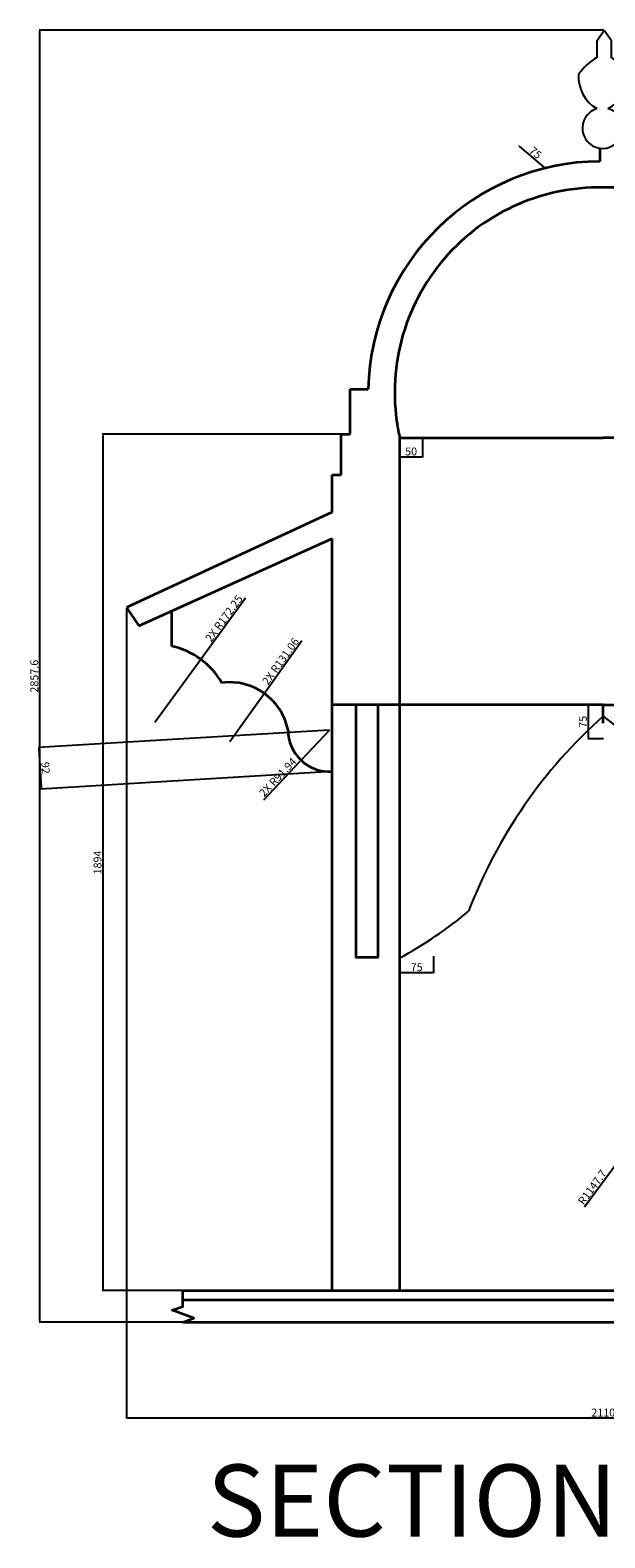
# Model space of a CAD drawing. Units: millimetres. Extents: x 498 to 8860, y -426 to 8717.
# Tile 5 of 9: x 527 to 1798, y 3606 to 6941. Entities that reach past the tile are written whole.
import ezdxf

# ---------------------------------------------------------------- set-up
doc = ezdxf.new("R2010")
doc.units = ezdxf.units.MM
for name, color, linetype, lineweight in [('A-ANNO-DIMS', 2, 'Continuous', 18), ('A-ANNO-TEXT', 3, 'Continuous', 18), ('A-DETL', 7, 'Continuous', 25), ('A-SECT', 7, 'Continuous', 35)]:
    doc.layers.add(name, color=color, linetype=linetype, lineweight=lineweight)
doc.styles.get("Standard").update_dxf_attribs({"font": 'arial.ttf'})
doc.dimstyles.new('ISO-25', dxfattribs={"dimtxt": 17.5, "dimasz": 2.5, "dimexe": 1.25, "dimexo": 0.625, "dimtad": 1, "dimdec": 0, "dimtxsty": 'Standard', "dimcen": 2.5, "dimadec": 0, "dimazin": 0, "dimtfac": 1, "dimtdec": 0, "dimtmove": 0, "dimatfit": 3, "dimfxl": 1, "dimarcsym": 0})

# ---------------------------------------------------------------- blocks, each defined once
blk = doc.blocks.new('*D29')
at = {"layer": 'A-ANNO-DIMS', "color": 0, "lineweight": -2, "transparency": 16777216}
for p, q in [((1344.7, 6038.9), (1344.7, 5996.1)), ((1394.8, 6038.9), (1394.8, 5996.1)), ((1347.2, 5997.3), (1392.3, 5997.3))]:
    blk.add_line(p, q, dxfattribs=at)
at = {"layer": 'A-ANNO-DIMS', "color": 0, "transparency": 16777216}
for points in [[(1347.2, 5997.8), (1347.2, 5996.9), (1344.7, 5997.3)], [(1392.3, 5997.8), (1392.3, 5996.9), (1394.8, 5997.3)]]:
    blk.add_solid(points, dxfattribs=at)
at = {"layer": 'Defpoints', "color": 0, "transparency": 16777216}
for p in [(1344.7, 6039.5), (1394.8, 6039.5), (1394.8, 5997.3)]:
    blk.add_point(p, dxfattribs=at)
at = {"layer": 'A-ANNO-DIMS', "color": 0, "transparency": 16777216, "insert": (1369.7, 6006.9), "char_height": 17.5, "attachment_point": 5}
blk.add_mtext('50', dxfattribs=at)
blk = doc.blocks.new('*D31')
at = {"layer": 'A-ANNO-DIMS', "color": 0, "lineweight": -2, "transparency": 16777216}
for p, q in [((1214.1, 6047.2), (686.4, 6047.2)), ((687.6, 6044.7), (687.6, 4155.7)), ((1194.1, 4153.2), (686.4, 4153.2))]:
    blk.add_line(p, q, dxfattribs=at)
at = {"layer": 'A-ANNO-DIMS', "color": 0, "transparency": 16777216}
for points in [[(687.2, 6044.7), (688, 6044.7), (687.6, 6047.2)], [(687.2, 4155.7), (688, 4155.7), (687.6, 4153.2)]]:
    blk.add_solid(points, dxfattribs=at)
at = {"layer": 'Defpoints', "color": 0, "transparency": 16777216}
for p in [(1214.7, 6047.2), (687.6, 4153.2), (1194.7, 4153.2)]:
    blk.add_point(p, dxfattribs=at)
at = {"layer": 'A-ANNO-DIMS', "color": 0, "transparency": 16777216, "insert": (678.1, 5100.2), "char_height": 17.5, "attachment_point": 5, "rotation": 90}
blk.add_mtext('1894', dxfattribs=at)
blk = doc.blocks.new('*D32')
at = {"layer": 'A-ANNO-DIMS', "color": 0, "lineweight": -2, "transparency": 16777216}
for p, q in [((1344.7, 4888.3), (1344.7, 4855.6)), ((1419.2, 4893), (1419.2, 4855.6)), ((1347.2, 4856.8), (1416.7, 4856.8))]:
    blk.add_line(p, q, dxfattribs=at)
at = {"layer": 'A-ANNO-DIMS', "color": 0, "transparency": 16777216}
for points in [[(1347.2, 4857.3), (1347.2, 4856.4), (1344.7, 4856.8)], [(1416.7, 4857.3), (1416.7, 4856.4), (1419.2, 4856.8)]]:
    blk.add_solid(points, dxfattribs=at)
at = {"layer": 'Defpoints', "color": 0, "transparency": 16777216}
for p in [(1344.7, 4889), (1419.2, 4893.6), (1419.2, 4856.8)]:
    blk.add_point(p, dxfattribs=at)
at = {"layer": 'A-ANNO-DIMS', "color": 0, "transparency": 16777216, "insert": (1382, 4866.4), "char_height": 17.5, "attachment_point": 5}
blk.add_mtext('75', dxfattribs=at)
blk = doc.blocks.new('*D34')
at = {"layer": 'A-ANNO-DIMS', "color": 0, "lineweight": -2, "transparency": 16777216}
for p, q in [((1794.1, 5448.8), (1760.3, 5448.8)), ((1761.6, 5446.3), (1761.6, 5376.5)), ((1795.1, 5374), (1760.3, 5374))]:
    blk.add_line(p, q, dxfattribs=at)
at = {"layer": 'A-ANNO-DIMS', "color": 0, "transparency": 16777216}
for points in [[(1761.2, 5446.3), (1762, 5446.3), (1761.6, 5448.8)], [(1761.2, 5376.5), (1762, 5376.5), (1761.6, 5374)]]:
    blk.add_solid(points, dxfattribs=at)
at = {"layer": 'Defpoints', "color": 0, "transparency": 16777216}
for p in [(1794.7, 5448.8), (1761.6, 5374), (1795.7, 5374)]:
    blk.add_point(p, dxfattribs=at)
at = {"layer": 'A-ANNO-DIMS', "color": 0, "transparency": 16777216, "insert": (1752, 5411.4), "char_height": 17.5, "attachment_point": 5, "rotation": 90}
blk.add_mtext('75', dxfattribs=at)
blk = doc.blocks.new('*D35')
at = {"layer": 'A-ANNO-DIMS', "color": 0, "lineweight": -2, "transparency": 16777216}
for p, q in [((1608, 6684.4), (1609.4, 6686)), ((1664.2, 6638.3), (1610.5, 6683.4)), ((1665.6, 6636.1), (1666.9, 6637.7))]:
    blk.add_line(p, q, dxfattribs=at)
at = {"layer": 'A-ANNO-DIMS', "color": 0, "transparency": 16777216}
for points in [[(1610.7, 6683.7), (1610.2, 6683.1), (1608.6, 6685)], [(1664.4, 6638.6), (1663.9, 6638), (1666.1, 6636.7)]]:
    blk.add_solid(points, dxfattribs=at)
at = {"layer": 'Defpoints', "color": 0, "transparency": 16777216}
for p in [(1607.6, 6683.9), (1608.6, 6685), (1665.2, 6635.6)]:
    blk.add_point(p, dxfattribs=at)
at = {"layer": 'A-ANNO-DIMS', "color": 0, "transparency": 16777216, "insert": (1643.4, 6668.2), "char_height": 17.5, "attachment_point": 5, "rotation": 319.9882}
blk.add_mtext('75', dxfattribs=at)
blk = doc.blocks.new('*D36')
at = {"layer": 'A-ANNO-DIMS', "color": 0, "lineweight": -2, "transparency": 16777216}
for p, q in [((1188.6, 5393.1), (545.2, 5354.5)), ((551.8, 5265.3), (546.6, 5352.1)), ((1194.1, 5301.3), (550.7, 5262.7))]:
    blk.add_line(p, q, dxfattribs=at)
at = {"layer": 'A-ANNO-DIMS', "color": 0, "transparency": 16777216}
for points in [[(547, 5352.1), (546.1, 5352.1), (546.4, 5354.6)], [(552.2, 5265.3), (551.3, 5265.3), (551.9, 5262.8)]]:
    blk.add_solid(points, dxfattribs=at)
at = {"layer": 'Defpoints', "color": 0, "transparency": 16777216}
for p in [(1189.2, 5393.1), (546.4, 5354.6), (1194.7, 5301.3)]:
    blk.add_point(p, dxfattribs=at)
at = {"layer": 'A-ANNO-DIMS', "color": 0, "transparency": 16777216, "insert": (558.7, 5309.3), "char_height": 17.5, "attachment_point": 5, "rotation": 273.429}
blk.add_mtext('92', dxfattribs=at)
blk = doc.blocks.new('FINIAL-BRASS')
for p, q in [((41.3, 239), (57, 261.6)), ((41.3, 202), (41.3, 239)), ((57, 261.6), (73.3, 238.5)), ((73.3, 199.9), (73.3, 238.5))]:
    blk.add_line(p, q)
for centre, radius, start, end in [((108.5, 89), 131.5, 120.7656, 145.5289), ((18.2, 106.2), 108.7, 31.7357, 59.5088), ((81.5, 158.5), 81.5, 176.5528, 239.9655), ((34.6, 158.5), 76.2, 293.2182, 3.7332), ((53.5, 44.9), 44.9, 106.5437, 75.6662)]:
    blk.add_arc(centre, radius, start, end)
blk = doc.blocks.new('BRACKET-STONE')
for centre, radius, start, end in [((1183.8, -291.1), 1104.6, 131.6209, 159.0769), ((-158.8, -276), 1013.9, 20.7397, 53.0882), ((-446.2, 819.4), 933, 298.5683, 309.875), ((1523.8, 965), 1147.7, 230.2129, 237.0762)]:
    blk.add_arc(centre, radius, start, end)
blk = doc.blocks.new('*D43')
at = {"layer": 'A-ANNO-DIMS', "color": 0, "lineweight": -2, "transparency": 16777216}
for p, q in [((739.8, 5663.4), (739.8, 3870.5)), ((2849.6, 5663.4), (2849.6, 3870.5)), ((742.3, 3871.8), (2847.1, 3871.8))]:
    blk.add_line(p, q, dxfattribs=at)
at = {"layer": 'A-ANNO-DIMS', "color": 0, "transparency": 16777216}
for points in [[(742.3, 3872.2), (742.3, 3871.3), (739.8, 3871.8)], [(2847.1, 3872.2), (2847.1, 3871.3), (2849.6, 3871.8)]]:
    blk.add_solid(points, dxfattribs=at)
at = {"layer": 'Defpoints', "color": 0, "transparency": 16777216}
for p in [(739.8, 5664), (2849.6, 5664), (2849.6, 3871.8)]:
    blk.add_point(p, dxfattribs=at)
at = {"layer": 'A-ANNO-DIMS', "color": 0, "transparency": 16777216, "insert": (1794.7, 3881.3), "char_height": 17.5, "attachment_point": 5}
blk.add_mtext('2110', dxfattribs=at)
blk = doc.blocks.new('*D44')
at = {"layer": 'A-ANNO-DIMS', "color": 0, "lineweight": -2, "transparency": 16777216}
for p, q in [((1796.4, 6941.1), (546.6, 6941.1)), ((547.8, 6938.6), (547.8, 4086)), ((864.1, 4083.5), (546.6, 4083.5))]:
    blk.add_line(p, q, dxfattribs=at)
at = {"layer": 'A-ANNO-DIMS', "color": 0, "transparency": 16777216}
for points in [[(547.4, 6938.6), (548.2, 6938.6), (547.8, 6941.1)], [(547.4, 4086), (548.2, 4086), (547.8, 4083.5)]]:
    blk.add_solid(points, dxfattribs=at)
at = {"layer": 'Defpoints', "color": 0, "transparency": 16777216}
for p in [(1797.1, 6941.1), (547.8, 4083.5), (864.7, 4083.5)]:
    blk.add_point(p, dxfattribs=at)
at = {"layer": 'A-ANNO-DIMS', "color": 0, "transparency": 16777216, "insert": (538.2, 5512.3), "char_height": 17.5, "attachment_point": 5, "rotation": 90}
blk.add_mtext('2857.6', dxfattribs=at)
blk = doc.blocks.new('*D76')
at = {"layer": 'A-ANNO-DIMS', "color": 0, "lineweight": -2, "transparency": 16777216}
for p, q in [((2868.5, 5853.9), (2188.2, 4929.6)), ((1753.1, 4338.5), (2186.7, 4927.6))]:
    blk.add_line(p, q, dxfattribs=at)
at = {"layer": 'A-ANNO-DIMS', "color": 0, "transparency": 16777216}
blk.add_solid([(2186.4, 4927.8), (2187.1, 4927.3), (2188.2, 4929.6)], dxfattribs=at)
at = {"layer": 'Defpoints', "color": 0, "transparency": 16777216}
for p in [(2868.5, 5853.9), (2188.2, 4929.6)]:
    blk.add_point(p, dxfattribs=at)
at = {"layer": 'A-ANNO-DIMS', "color": 0, "transparency": 16777216, "insert": (1772.4, 4380.6), "char_height": 17.5, "attachment_point": 5, "rotation": 53.6461}
blk.add_mtext('R1147.7', dxfattribs=at)
blk = doc.blocks.new('*D77')
at = {"layer": 'A-ANNO-DIMS', "color": 0, "lineweight": -2, "transparency": 16777216}
for p, q in [((1003.2, 5684.9), (905.6, 5551.6)), ((802.3, 5410.7), (904.1, 5549.6))]:
    blk.add_line(p, q, dxfattribs=at)
at = {"layer": 'A-ANNO-DIMS', "color": 0, "transparency": 16777216}
blk.add_solid([(905.3, 5551.9), (905.9, 5551.4), (904.1, 5549.6)], dxfattribs=at)
at = {"layer": 'Defpoints', "color": 0, "transparency": 16777216}
for p in [(904.1, 5549.6), (802.3, 5410.7)]:
    blk.add_point(p, dxfattribs=at)
at = {"layer": 'A-ANNO-DIMS', "color": 0, "transparency": 16777216, "insert": (957.5, 5638.6), "char_height": 17.5, "attachment_point": 5, "rotation": 53.7735}
blk.add_mtext('2X R172.25', dxfattribs=at)
blk = doc.blocks.new('*D78')
at = {"layer": 'A-ANNO-DIMS', "color": 0, "lineweight": -2, "transparency": 16777216}
for p, q in [((1128, 5590.6), (1046.4, 5476.4)), ((968.7, 5367.7), (1044.9, 5474.3))]:
    blk.add_line(p, q, dxfattribs=at)
at = {"layer": 'A-ANNO-DIMS', "color": 0, "transparency": 16777216}
blk.add_solid([(1046, 5476.6), (1046.7, 5476.1), (1044.9, 5474.3)], dxfattribs=at)
at = {"layer": 'Defpoints', "color": 0, "transparency": 16777216}
for p in [(1044.9, 5474.3), (968.7, 5367.7)]:
    blk.add_point(p, dxfattribs=at)
at = {"layer": 'A-ANNO-DIMS', "color": 0, "transparency": 16777216, "insert": (1082.8, 5543.9), "char_height": 17.5, "attachment_point": 5, "rotation": 54.4526}
blk.add_mtext('2X R131.06', dxfattribs=at)
blk = doc.blocks.new('*D79')
at = {"layer": 'A-ANNO-DIMS', "color": 0, "lineweight": -2, "transparency": 16777216}
for p, q in [((1189.2, 5393.1), (1126.2, 5326.2)), ((1044, 5238.9), (1124.5, 5324.4))]:
    blk.add_line(p, q, dxfattribs=at)
at = {"layer": 'A-ANNO-DIMS', "color": 0, "transparency": 16777216}
blk.add_solid([(1124.2, 5324.7), (1124.8, 5324.1), (1126.2, 5326.2)], dxfattribs=at)
at = {"layer": 'Defpoints', "color": 0, "transparency": 16777216}
for p in [(1189.2, 5393.1), (1126.2, 5326.2)]:
    blk.add_point(p, dxfattribs=at)
at = {"layer": 'A-ANNO-DIMS', "color": 0, "transparency": 16777216, "insert": (1076.4, 5287.3), "char_height": 17.5, "attachment_point": 5, "rotation": 46.7142}
blk.add_mtext('2X R91.94', dxfattribs=at)

msp = doc.modelspace()

# ---------------------------------------------------------------- linework, layer by layer
at = {"layer": 'A-SECT'}
for p, q in [((1787.151, 6679.961), (1787.151, 6650.915)), ((1234.726, 6047.245), (1234.726, 6147.245)), ((1234.726, 6147.245), (1274.726, 6147.245)), ((1214.726, 5957.887), (1214.726, 6047.245)), ((1214.726, 6047.245), (1234.726, 6047.245)), ((1344.726, 5448.755), (1344.726, 6039.541)), ((1344.726, 6039.541), (1794.726, 6039.541)), ((2244.726, 6039.541), (1794.726, 6039.541)), ((1194.726, 5875.163), (1194.726, 5957.887)), ((1194.726, 5957.887), (1214.726, 5957.887)), ((1194.726, 5875.163), (739.808, 5663.993)), ((767.153, 5623.74), (1194.726, 5817.007)), ((1194.726, 5448.755), (1194.726, 5817.007)), ((739.808, 5663.993), (767.153, 5623.74)), ((840.334, 5578.673), (840.334, 5656.819)), ((1194.726, 4153.169), (1194.726, 5448.755)), ((1794.726, 5448.755), (1194.726, 5448.755)), ((1344.726, 4153.169), (1344.726, 5448.755)), ((1794.726, 5448.755), (2394.726, 5448.755)), ((1794.872, 5408.235), (1794.726, 5448.755)), ((864.726, 4153.169), (2724.726, 4153.169)), ((864.726, 4133.169), (2724.726, 4133.169)), ((864.726, 4083.169), (2724.726, 4083.169))]:
    msp.add_line(p, q, dxfattribs=at)
msp.add_lwpolyline([(1296.443, 5448.755), (1247.099, 5448.755), (1247.099, 4890.556), (1296.443, 4890.556)], close=True, dxfattribs=at)
msp.add_lwpolyline([(864.726, 4083.169), (864.726, 4083.522), (888.695, 4092.246), (840.757, 4109.694), (864.726, 4118.419), (864.726, 4153.169)], dxfattribs=at)
for centre, radius, start, end in [((1789.885, 6135.632), 515.29, 90.304093, 178.708663), ((1786.134, 6140.339), 452.771, 88.912714, 192.86325), ((1803.318, 6140.339), 452.771, 347.13675, 91.087286), ((802.318, 5410.667), 172.253, 30.289705, 77.249938), ((968.72, 5367.687), 131.056, 11.188127, 97.745996), ((1189.227, 5393.116), 91.941, 180, 273.429009)]:
    msp.add_arc(centre, radius, start, end, dxfattribs=at)

# ---------------------------------------------------------------- block references
at = {"layer": 'A-DETL'}
for name, p in [('FINIAL-BRASS', (1740.051, 6679.509)), ('BRACKET-STONE', (1344.726, 4888.954))]:
    msp.add_blockref(name, p, dxfattribs=at)

# ---------------------------------------------------------------- texts
at = {"layer": 'A-ANNO-TEXT'}
msp.add_text('SECTION AT X-X', height=159.20004, dxfattribs=at).set_placement((917.853, 3609.29))

# ---------------------------------------------------------------- dimensions: what is measured, and where the dimension line sits
at = {"layer": 'A-ANNO-DIMS'}
for base, p1, p2, override, picture, middle in [((547.808, 4083.522), (1797.055, 6941.084), (864.726, 4083.522), {"dimdec": 1, "dimlfac": 1, "dimrnd": 0, "dimzin": 0, "dimdsep": 46, "dimlunit": 2}, '*D44', (538.247, 5512.303)), ((687.632, 4153.169), (1214.726, 6047.245), (1194.726, 4153.169), {"dimclrd": 0, "dimclre": 0, "dimclrt": 0}, '*D31', (678.072, 5100.207)), ((1761.573, 5374.049), (1794.726, 5448.755), (1795.719, 5374.049), {"dimclrd": 0, "dimclre": 0, "dimclrt": 0}, '*D34', (1752.049, 5411.402))]:
    dim = msp.add_linear_dim(base=base, p1=p1, p2=p2, angle=90, dimstyle='ISO-25', override=override, dxfattribs=at)
    dim.commit()
    dim.dimension.update_dxf_attribs({"geometry": picture, "text_midpoint": middle})
for p1, p2, distance, picture, middle in [((1665.154, 6635.598), (1607.622, 6683.894), -1.458, '*D35', (1643.449, 6668.158)), ((1194.726, 5301.339), (1189.227, 5393.116), 643.973, '*D36', (558.699, 5309.282))]:
    dim = msp.add_aligned_dim(p1=p1, p2=p2, distance=distance, dimstyle='ISO-25', override={"dimclrd": 0, "dimclre": 0, "dimclrt": 0}, dxfattribs=at)
    dim.commit()
    dim.dimension.update_dxf_attribs({"geometry": picture, "text_midpoint": middle})
for base, p1, p2, override, picture, middle in [((1394.771, 5997.344), (1344.726, 6039.541), (1394.771, 6039.541), {"dimclrd": 0, "dimclre": 0, "dimclrt": 0}, '*D29', (1369.749, 6006.904)), ((2849.644, 3871.756), (739.808, 5663.993), (2849.644, 5663.993), {"dimdec": 0, "dimlfac": 1, "dimrnd": 0, "dimzin": 0, "dimdsep": 46, "dimlunit": 2}, '*D43', (1794.726, 3881.316)), ((1419.241, 4856.836), (1344.726, 4888.954), (1419.241, 4893.609), {"dimclrd": 0, "dimclre": 0, "dimclrt": 0}, '*D32', (1381.984, 4866.36))]:
    dim = msp.add_linear_dim(base=base, p1=p1, p2=p2, dimstyle='ISO-25', override=override, dxfattribs=at)
    dim.commit()
    dim.dimension.update_dxf_attribs({"geometry": picture, "text_midpoint": middle})
dim = msp.add_radius_dim(center=(2868.528, 5853.93), mpoint=(2188.204, 4929.605), dimstyle='ISO-25', override={"dimdec": 1, "dimlfac": 1, "dimrnd": 0, "dimzin": 0, "dimdsep": 46, "dimlunit": 2}, dxfattribs=at)
dim.commit()
dim.dimension.update_dxf_attribs({"geometry": '*D76', "text_midpoint": (1780.009, 4375.01), "dimtype": 164})
for center, mpoint, picture, middle in [((802.318, 5410.667), (904.116, 5549.622), '*D77', (965.195, 5632.994)), ((968.72, 5367.687), (1044.913, 5474.319), '*D78', (1090.629, 5538.298))]:
    dim = msp.add_radius_dim(center=center, mpoint=mpoint, text='2X <>', dimstyle='ISO-25', override={"dimdec": 2, "dimlfac": 1, "dimrnd": 0, "dimzin": 0, "dimdsep": 46, "dimlunit": 2}, dxfattribs=at)
    dim.commit()
    dim.dimension.update_dxf_attribs({"geometry": picture, "text_midpoint": middle, "dimtype": 164})
dim = msp.add_radius_dim(center=(1189.227, 5393.116), mpoint=(1126.189, 5326.188), text='2X <>', dimstyle='ISO-25', override={"dimdec": 2, "dimlfac": 1, "dimrnd": 0, "dimzin": 0, "dimdsep": 46, "dimlunit": 2}, dxfattribs=at)
dim.commit()
dim.dimension.update_dxf_attribs({"geometry": '*D79', "text_midpoint": (1076.418, 5287.29)})

doc.saveas('drawing.dxf')
